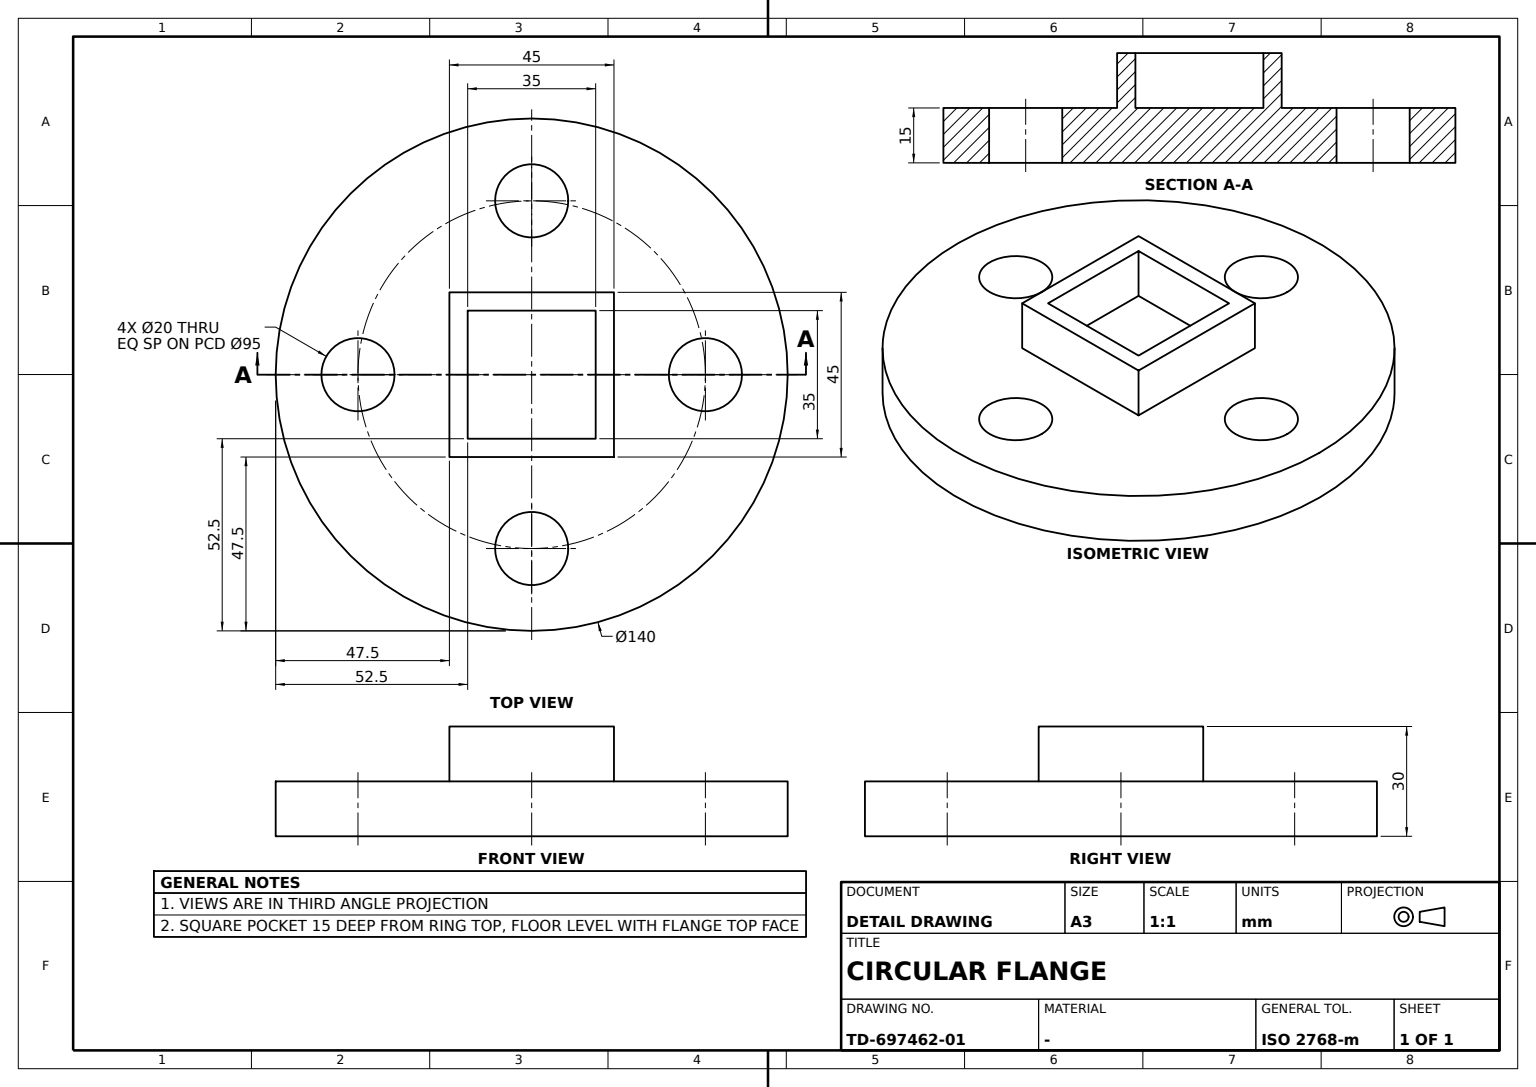
CATIA V5 part; units mm, degrees
sketch "Sketch1" plane through (0, 0, 0) normal (0, 0, 1) x (1, 0, 0)
  circle A0 centre (0, 0) radius 70
  dimension "radius A0" = 70
extrude "Pad1" add sketch "Sketch1" along normal blind 15
sketch "Sketch2" plane through (0, 0, 15) normal (0, 0, 1) x (1, 0, 0)
  circle A0 centre (0, 0) radius 47.5 construction
  circle A1 centre (0, 47.5) radius 10
  point P0 (0, 47.5)
  circle A2 centre (47.5, 0) radius 10
  point P1 (47.5, 0)
  circle A3 centre (-47.5, 0) radius 10
  point P2 (-47.5, 0)
  circle A4 centre (0, -47.5) radius 10
  point P3 (0, -47.5)
  dimension "radius A0" = 47.5
  dimension "radius A1" = 10
  dimension "radius A2" = 10
  dimension "radius A4" = 10
  dimension "radius A3" = 10
  constraint coincidence P0 A0
  constraint coincidence P1 A0
  constraint coincidence P1 x-axis
  constraint coincidence P2 A0
  constraint coincidence P2 x-axis
  constraint coincidence P3 A0
  constraint coincidence P3 y-axis
  constraint coincidence P0 y-axis
extrude "Pocket1" cut sketch "Sketch2" against normal blind 15
sketch "Sketch3" plane through (0, 0, 15) normal (0, 0, 1) x (1, 0, 0)
  line L0 (17.5, 17.5) -> (17.5, -17.5)
  line L1 (17.5, -17.5) -> (-17.5, -17.5)
  line L2 (-17.5, -17.5) -> (-17.5, 17.5)
  line L3 (-17.5, 17.5) -> (17.5, 17.5)
  line L4 (22.5, 22.5) -> (22.5, -22.5)
  line L5 (22.5, -22.5) -> (-22.5, -22.5)
  line L6 (-22.5, -22.5) -> (-22.5, 22.5)
  line L7 (-22.5, 22.5) -> (22.5, 22.5)
  dimension "length L7" = 45
  dimension "distance L5 L7" = 45
  dimension "length L3" = 35
  dimension "distance L1 L3" = 35
  constraint vertical L0 y-axis
  constraint vertical L2 y-axis
  constraint vertical L4 y-axis
  constraint vertical L6 y-axis
  constraint horizontal L1 x-axis
  constraint horizontal L3 x-axis
  constraint horizontal L5 x-axis
  constraint horizontal L7 x-axis
  constraint equidistance L0 L2 origin
  constraint equidistance L1 L3 origin
  constraint equidistance L4 L6 origin
  constraint equidistance L5 L7 origin
extrude "Pad2" add sketch "Sketch3" along normal blind 15
